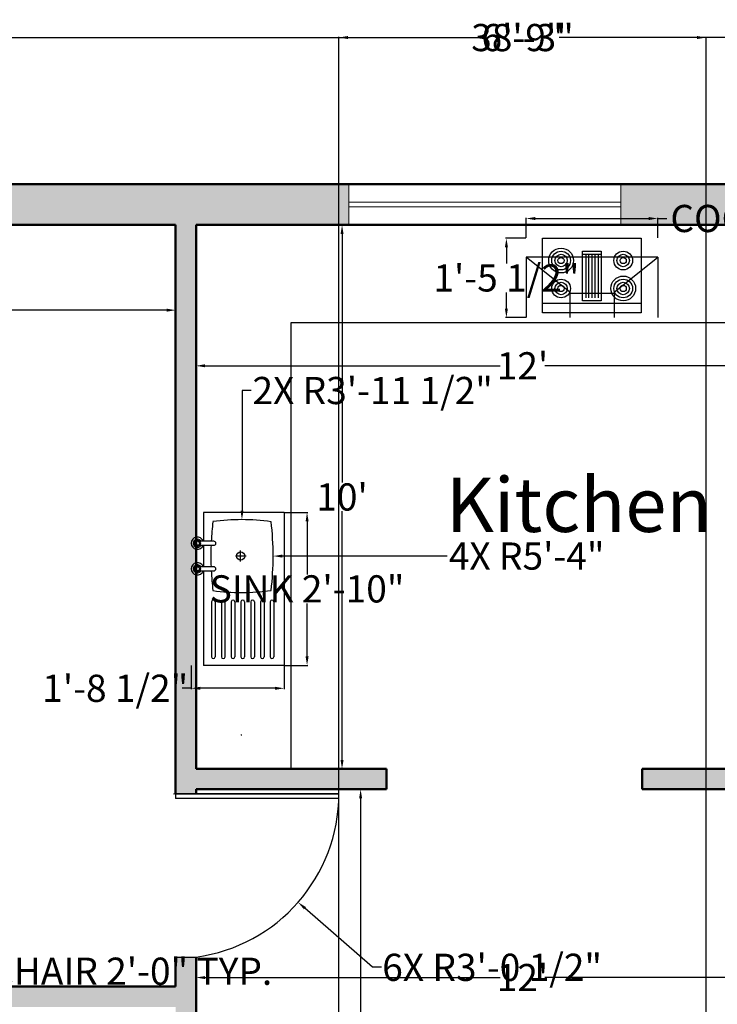
# Model space of a CAD drawing. Units: inches. Extents: x 2436 to 2989, y 5527 to 6207.
# Tile 4 of 5: x 2605 to 2759, y 5989 to 6207. Entities that reach past the tile are written whole.
import ezdxf

# ---------------------------------------------------------------- set-up
doc = ezdxf.new("R2010")
doc.units = ezdxf.units.IN
doc.header["$MEASUREMENT"] = 0
for name, color, linetype, lineweight in [('A-ANNO-DIMS', 2, 'Continuous', 18), ('A-AREA-IDEN', 7, 'Continuous', 25), ('A-DOOR', 3, 'Continuous', 25), ('A-EQPM', 8, 'Continuous', 25), ('A-FLOR-CASE', 9, 'Continuous', 25), ('A-FLOR-FIXT', 8, 'Continuous', 25), ('A-GLAZ', 4, 'Continuous', 18), ('A-WALL', 7, 'Continuous', 50), ('A-WALL-PATT', 252, 'Continuous', 13)]:
    doc.layers.add(name, color=color, linetype=linetype, lineweight=lineweight)
doc.styles.get("Standard").update_dxf_attribs({"font": 'arial.ttf'})
doc.dimstyles.get("Standard").update_dxf_attribs({"dimtxt": 6, "dimasz": 2, "dimexe": 0.18, "dimexo": 0.0625, "dimgap": 0.09, "dimtad": 0, "dimtih": 1, "dimtoh": 1, "dimdec": 0, "dimzin": 0, "dimdsep": 46, "dimlunit": 3, "dimtxsty": 'Standard', "dimcen": 0.09, "dimadec": 0, "dimazin": 0, "dimtfac": 1, "dimtdec": 0, "dimtofl": 0, "dimtmove": 0, "dimatfit": 3, "dimfxl": 1, "dimtolj": 1, "dimtzin": 0, "dimarcsym": 0})

# ---------------------------------------------------------------- blocks, each defined once
blk = doc.blocks.new('*D4')
at = {"layer": 'A-ANNO-DIMS', "color": 0, "lineweight": -2, "transparency": 16777216}
for p, q in [((2495.39, 6161.17), (2495.39, 6142.26)), ((2639.39, 6161.17), (2639.39, 6142.26)), ((2497.39, 6142.44), (2562.49, 6142.44)), ((2637.39, 6142.44), (2572.29, 6142.44))]:
    blk.add_line(p, q, dxfattribs=at)
at = {"layer": 'A-ANNO-DIMS', "color": 0, "transparency": 16777216}
for points in [[(2497.39, 6142.77), (2497.39, 6142.1), (2495.39, 6142.44)], [(2637.39, 6142.77), (2637.39, 6142.1), (2639.39, 6142.44)]]:
    blk.add_solid(points, dxfattribs=at)
at = {"layer": 'Defpoints', "color": 0, "transparency": 16777216}
for p in [(2495.39, 6161.23), (2639.39, 6161.23), (2639.39, 6142.44)]:
    blk.add_point(p, dxfattribs=at)
at = {"layer": 'A-ANNO-DIMS', "color": 0, "transparency": 16777216, "insert": (2567.39, 6142.44), "char_height": 6, "attachment_point": 5}
blk.add_mtext("\\A1;12'", dxfattribs=at)
blk = doc.blocks.new('*D5')
at = {"layer": 'A-ANNO-DIMS', "color": 0, "lineweight": -2, "transparency": 16777216}
for p, q in [((2643.89, 6161.17), (2643.89, 6129.98)), ((2787.89, 6161.17), (2787.89, 6129.98)), ((2645.89, 6130.16), (2710.99, 6130.16)), ((2785.89, 6130.16), (2720.79, 6130.16))]:
    blk.add_line(p, q, dxfattribs=at)
at = {"layer": 'A-ANNO-DIMS', "color": 0, "transparency": 16777216}
for points in [[(2645.89, 6130.5), (2645.89, 6129.83), (2643.89, 6130.16)], [(2785.89, 6130.5), (2785.89, 6129.83), (2787.89, 6130.16)]]:
    blk.add_solid(points, dxfattribs=at)
at = {"layer": 'Defpoints', "color": 0, "transparency": 16777216}
for p in [(2643.89, 6161.23), (2787.89, 6161.23), (2787.89, 6130.16)]:
    blk.add_point(p, dxfattribs=at)
at = {"layer": 'A-ANNO-DIMS', "color": 0, "transparency": 16777216, "insert": (2715.89, 6130.16), "char_height": 6, "attachment_point": 5}
blk.add_mtext("\\A1;12'", dxfattribs=at)
blk = doc.blocks.new('*D6')
at = {"layer": 'A-ANNO-DIMS', "color": 0, "lineweight": -2, "transparency": 16777216}
for p, q in [((2643.95, 6161.23), (2676.27, 6161.23)), ((2676.09, 6159.23), (2676.09, 6104.39)), ((2676.09, 6043.23), (2676.09, 6098.08)), ((2643.95, 6041.23), (2676.27, 6041.23))]:
    blk.add_line(p, q, dxfattribs=at)
at = {"layer": 'A-ANNO-DIMS', "color": 0, "transparency": 16777216}
for points in [[(2675.76, 6159.23), (2676.43, 6159.23), (2676.09, 6161.23)], [(2675.76, 6043.23), (2676.43, 6043.23), (2676.09, 6041.23)]]:
    blk.add_solid(points, dxfattribs=at)
at = {"layer": 'Defpoints', "color": 0, "transparency": 16777216}
for p in [(2643.89, 6161.23), (2643.89, 6041.23), (2676.09, 6041.23)]:
    blk.add_point(p, dxfattribs=at)
at = {"layer": 'A-ANNO-DIMS', "color": 0, "transparency": 16777216, "insert": (2676.09, 6101.23), "char_height": 6, "attachment_point": 5}
blk.add_mtext("\\A1;10'", dxfattribs=at)
blk = doc.blocks.new('*D19')
at = {"layer": 'A-ANNO-DIMS', "color": 0, "lineweight": -2, "transparency": 16777216}
for p, q in [((2667.17, 6036.73), (2680.37, 6036.73)), ((2680.19, 6034.73), (2680.19, 5949.89)), ((2680.19, 5858.73), (2680.19, 5943.58)), ((2667.17, 5856.73), (2680.37, 5856.73))]:
    blk.add_line(p, q, dxfattribs=at)
at = {"layer": 'A-ANNO-DIMS', "color": 0, "transparency": 16777216}
for points in [[(2679.86, 6034.73), (2680.52, 6034.73), (2680.19, 6036.73)], [(2679.86, 5858.73), (2680.52, 5858.73), (2680.19, 5856.73)]]:
    blk.add_solid(points, dxfattribs=at)
at = {"layer": 'Defpoints', "color": 0, "transparency": 16777216}
for p in [(2667.11, 6036.73), (2667.11, 5856.73), (2680.19, 5856.73)]:
    blk.add_point(p, dxfattribs=at)
at = {"layer": 'A-ANNO-DIMS', "color": 0, "transparency": 16777216, "insert": (2680.19, 5946.73), "char_height": 6, "attachment_point": 5}
blk.add_mtext("\\A1;15'", dxfattribs=at)
blk = doc.blocks.new('*D20')
at = {"layer": 'A-ANNO-DIMS', "color": 0, "lineweight": -2, "transparency": 16777216}
for p, q in [((2643.89, 5989.83), (2643.89, 5995.38)), ((2787.89, 5989.83), (2787.89, 5995.38)), ((2645.89, 5995.2), (2710.99, 5995.2)), ((2785.89, 5995.2), (2720.79, 5995.2))]:
    blk.add_line(p, q, dxfattribs=at)
at = {"layer": 'A-ANNO-DIMS', "color": 0, "transparency": 16777216}
for points in [[(2645.89, 5995.53), (2645.89, 5994.87), (2643.89, 5995.2)], [(2785.89, 5995.53), (2785.89, 5994.87), (2787.89, 5995.2)]]:
    blk.add_solid(points, dxfattribs=at)
at = {"layer": 'Defpoints', "color": 0, "transparency": 16777216}
for p in [(2787.89, 5995.2), (2643.89, 5989.77), (2787.89, 5989.77)]:
    blk.add_point(p, dxfattribs=at)
at = {"layer": 'A-ANNO-DIMS', "color": 0, "transparency": 16777216, "insert": (2715.89, 5995.2), "char_height": 6, "attachment_point": 5}
blk.add_mtext("\\A1;12'", dxfattribs=at)
blk = doc.blocks.new('chimmne')
for p, q in [((17.89, 6.07), (-18.11, 6.07)), ((-18.11, 6.07), (-18.11, -10.43)), ((-6.16, -3.43), (-18.11, 6.07)), ((5.94, -3.43), (17.89, 6.07)), ((17.89, 6.07), (17.89, -10.43)), ((-6.16, -3.43), (-6.16, -10.43)), ((5.94, -3.82), (-6.16, -3.82)), ((5.94, -3.43), (5.94, -10.43))]:
    blk.add_line(p, q)
for points in [[(-13.61, -9.12), (-13.61, 11.28), (13.39, 11.28), (13.39, -9.12)], [(-2.66, -5.87), (-2.66, 7.73), (2.44, 7.73), (2.44, -5.87)]]:
    blk.add_lwpolyline(points, close=True)
for points in [[(-2.66, 6.88), (2.44, 6.88)], [(-1.81, 6.88), (-1.81, -5.02)], [(-0.96, -5.02), (-0.96, 6.88)], [(-0.11, 6.88), (-0.11, -5.02)], [(0.74, -5.02), (0.74, 6.88)], [(1.59, 6.88), (1.59, -5.02)], [(13.39, -6.57), (-13.61, -6.57)]]:
    blk.add_lwpolyline(points)
for centre, radius in [((-8.55, 5.18), 3.4), ((-8.55, 5.18), 2.55), ((-8.55, 5.18), 1.7), ((-8.55, 5.18), 0.85), ((8.44, 5.18), 2.55), ((8.44, 5.18), 1.7), ((8.44, 5.18), 0.85), ((-8.55, -2.47), 2.55), ((8.44, -2.47), 3.4), ((8.44, -2.47), 2.55), ((-8.55, -2.47), 1.7), ((-8.55, -2.47), 0.85), ((8.44, -2.47), 1.7), ((8.44, -2.47), 0.85)]:
    blk.add_circle(centre, radius)
blk = doc.blocks.new('A$C799204C7')
for p, q in [((0, 34.2), (17.99, 34.2)), ((0, 0), (0, 34.2)), ((17.99, 13.08), (17.99, 34.2)), ((2.32, 20.01), (2.32, 32.27)), ((3.13, 20.01), (3.13, 32.27)), ((4.48, 20.01), (4.48, 32.27)), ((5.29, 20.01), (5.29, 32.27)), ((6.64, 20.01), (6.64, 32.27)), ((7.45, 20.01), (7.45, 32.27)), ((8.85, 20.01), (8.85, 32.27)), ((9.66, 20.01), (9.66, 32.27)), ((11.01, 20.01), (11.01, 32.27)), ((11.82, 20.01), (11.82, 32.27)), ((13.22, 20.01), (13.22, 32.27)), ((14.03, 20.01), (14.03, 32.27)), ((15.42, 20.01), (15.42, 32.27)), ((16.24, 20.01), (16.24, 32.27)), ((18.59, 13.08), (15.71, 13.08)), ((15.71, 12.17), (18.59, 12.17)), ((17.99, 7.36), (17.99, 12.17)), ((8.52, 9.77), (10.9, 9.77)), ((9.73, 11), (9.73, 8.54)), ((18.59, 7.36), (15.71, 7.36)), ((15.71, 6.45), (18.59, 6.45)), ((17.99, 0), (17.99, 6.45)), ((0, 0), (17.99, 0))]:
    blk.add_line(p, q)
for centre, radius in [((19.38, 12.62), 0.684), ((19.38, 12.62), 0.456), ((9.7, 9.77), 0.916), ((19.38, 6.91), 0.684), ((19.38, 6.91), 0.456)]:
    blk.add_circle(centre, radius)
for centre, radius, start, end in [((2.72, 32.27), 0.407, 0, 180), ((4.88, 32.27), 0.407, 0, 180), ((7.05, 32.27), 0.407, 0, 180), ((9.25, 32.27), 0.407, 0, 180), ((11.42, 32.27), 0.407, 0, 180), ((13.62, 32.27), 0.407, 0, 180), ((15.83, 32.27), 0.407, 0, 180), ((2.72, 20.01), 0.407, 180, 0), ((4.88, 20.01), 0.407, 180, 0), ((7.05, 20.01), 0.407, 180, 0), ((9.25, 20.01), 0.407, 180, 0), ((11.42, 20.01), 0.407, 180, 0), ((13.62, 20.01), 0.407, 180, 0), ((15.83, 20.01), 0.407, 180, 0), ((9.53, -30.19), 48.1, 82.3437, 97.8966), ((67.33, 9.77), 64.88, 173.1952, 186.8048), ((-48.51, 9.77), 64.88, 2.9208, 6.8048), ((19.38, 12.62), 1.37, 199.6514, 160.3603), ((19.38, 12.62), 0.911, 210.3431, 149.7554), ((15.71, 12.62), 0.456, 90, 270), ((-48.51, 9.77), 64.88, 357.8723, 2.115), ((15.71, 6.91), 0.456, 90, 270), ((19.38, 6.91), 1.37, 199.6514, 160.3603), ((19.38, 6.91), 0.911, 210.3431, 149.7554), ((-48.51, 9.77), 64.88, 353.1952, 357.0665), ((9.53, 49.73), 48.1, 262.1034, 277.6563)]:
    blk.add_arc(centre, radius, start, end)
blk = doc.blocks.new('WINDOW-60IN')
for p, q in [((0, 9), (0, 0)), ((60, 9), (0, 9)), ((60, 0), (60, 9)), ((60, 5), (0, 5)), ((0, 4), (60, 4)), ((0, 0), (60, 0))]:
    blk.add_line(p, q)
blk = doc.blocks.new('*D34')
at = {"layer": 'A-ANNO-DIMS', "color": 0, "lineweight": -2, "transparency": 16777216}
for p, q in [((2553.14, 6000.14), (2553.14, 5996.42)), ((2577.11, 6000.14), (2577.11, 5996.42)), ((2555.14, 5996.6), (2575.11, 5996.6)), ((2577.11, 5996.6), (2579.11, 5996.6))]:
    blk.add_line(p, q, dxfattribs=at)
at = {"layer": 'A-ANNO-DIMS', "color": 0, "transparency": 16777216}
for points in [[(2555.14, 5996.94), (2555.14, 5996.27), (2553.14, 5996.6)], [(2575.11, 5996.94), (2575.11, 5996.27), (2577.11, 5996.6)]]:
    blk.add_solid(points, dxfattribs=at)
at = {"layer": 'Defpoints', "color": 0, "transparency": 16777216}
for p in [(2553.14, 6000.2), (2577.11, 6000.2), (2577.11, 5996.6)]:
    blk.add_point(p, dxfattribs=at)
at = {"layer": 'A-ANNO-DIMS', "color": 0, "transparency": 16777216, "insert": (2621.18, 5996.6), "char_height": 6, "attachment_point": 5}
blk.add_mtext('\\A1;ARMCHAIR 2\'-0" TYP.', dxfattribs=at)
blk = doc.blocks.new('*D44')
at = {"layer": 'A-ANNO-DIMS', "color": 0, "lineweight": -2, "transparency": 16777216}
for p, q in [((2716.7, 6158.37), (2716.7, 6162.84)), ((2718.7, 6162.66), (2743.72, 6162.66)), ((2745.72, 6158.37), (2745.72, 6162.84)), ((2745.72, 6162.66), (2747.72, 6162.66))]:
    blk.add_line(p, q, dxfattribs=at)
at = {"layer": 'A-ANNO-DIMS', "color": 0, "transparency": 16777216}
for points in [[(2718.7, 6162.99), (2718.7, 6162.32), (2716.7, 6162.66)], [(2743.72, 6162.99), (2743.72, 6162.32), (2745.72, 6162.66)]]:
    blk.add_solid(points, dxfattribs=at)
at = {"layer": 'Defpoints', "color": 0, "transparency": 16777216}
for p in [(2745.72, 6162.66), (2716.7, 6158.3), (2745.72, 6158.3)]:
    blk.add_point(p, dxfattribs=at)
at = {"layer": 'A-ANNO-DIMS', "color": 0, "transparency": 16777216, "insert": (2777.87, 6162.66), "char_height": 6, "attachment_point": 5}
blk.add_mtext('\\A1;COOKTOP 2\'-5"', dxfattribs=at)
blk = doc.blocks.new('*D45')
at = {"layer": 'A-ANNO-DIMS', "color": 0, "lineweight": -2, "transparency": 16777216}
for p, q in [((2716.63, 6158.3), (2712.16, 6158.3)), ((2712.34, 6156.3), (2712.34, 6152.75)), ((2712.34, 6142.8), (2712.34, 6146.36)), ((2716.63, 6140.8), (2712.16, 6140.8))]:
    blk.add_line(p, q, dxfattribs=at)
at = {"layer": 'A-ANNO-DIMS', "color": 0, "transparency": 16777216}
for points in [[(2712.01, 6156.3), (2712.68, 6156.3), (2712.34, 6158.3)], [(2712.01, 6142.8), (2712.68, 6142.8), (2712.34, 6140.8)]]:
    blk.add_solid(points, dxfattribs=at)
at = {"layer": 'Defpoints', "color": 0, "transparency": 16777216}
for p in [(2712.34, 6158.3), (2716.7, 6158.3), (2716.7, 6140.8)]:
    blk.add_point(p, dxfattribs=at)
at = {"layer": 'A-ANNO-DIMS', "color": 0, "transparency": 16777216, "insert": (2712.34, 6149.55), "char_height": 6, "attachment_point": 5}
blk.add_mtext('\\A1;1\'-5 1/2"', dxfattribs=at)
blk = doc.blocks.new('*D46')
at = {"layer": 'A-ANNO-DIMS', "color": 0, "lineweight": -2, "transparency": 16777216}
for p, q in [((2663.38, 6097.83), (2668.56, 6097.83)), ((2668.38, 6095.83), (2668.38, 6084.15)), ((2668.38, 6066.08), (2668.38, 6077.76)), ((2663.38, 6064.08), (2668.56, 6064.08))]:
    blk.add_line(p, q, dxfattribs=at)
at = {"layer": 'A-ANNO-DIMS', "color": 0, "transparency": 16777216}
for points in [[(2668.05, 6095.83), (2668.72, 6095.83), (2668.38, 6097.83)], [(2668.05, 6066.08), (2668.72, 6066.08), (2668.38, 6064.08)]]:
    blk.add_solid(points, dxfattribs=at)
at = {"layer": 'Defpoints', "color": 0, "transparency": 16777216}
for p in [(2663.32, 6097.83), (2663.32, 6064.08), (2668.38, 6064.08)]:
    blk.add_point(p, dxfattribs=at)
at = {"layer": 'A-ANNO-DIMS', "color": 0, "transparency": 16777216, "insert": (2668.38, 6080.95), "char_height": 6, "attachment_point": 5}
blk.add_mtext('\\A1;SINK 2\'-10"', dxfattribs=at)
blk = doc.blocks.new('*D47')
at = {"layer": 'A-ANNO-DIMS', "color": 0, "lineweight": -2, "transparency": 16777216}
for p, q in [((2642.85, 6064.02), (2642.85, 6058.84)), ((2663.32, 6064.02), (2663.32, 6058.84)), ((2642.85, 6059.02), (2640.85, 6059.02)), ((2661.32, 6059.02), (2644.85, 6059.02))]:
    blk.add_line(p, q, dxfattribs=at)
at = {"layer": 'A-ANNO-DIMS', "color": 0, "transparency": 16777216}
for points in [[(2644.85, 6059.35), (2644.85, 6058.68), (2642.85, 6059.02)], [(2661.32, 6059.35), (2661.32, 6058.68), (2663.32, 6059.02)]]:
    blk.add_solid(points, dxfattribs=at)
at = {"layer": 'Defpoints', "color": 0, "transparency": 16777216}
for p in [(2642.85, 6064.08), (2663.32, 6064.08), (2642.85, 6059.02)]:
    blk.add_point(p, dxfattribs=at)
at = {"layer": 'A-ANNO-DIMS', "color": 0, "transparency": 16777216, "insert": (2626.07, 6059.02), "char_height": 6, "attachment_point": 5}
blk.add_mtext('\\A1;1\'-8 1/2"', dxfattribs=at)
blk = doc.blocks.new('*D48')
at = {"layer": 'A-ANNO-DIMS', "color": 0, "lineweight": -2, "transparency": 16777216}
for p, q in [((2486.39, 6170.29), (2486.39, 6202.76)), ((2488.39, 6202.58), (2705.49, 6202.58)), ((2943.39, 6202.58), (2726.28, 6202.58)), ((2945.39, 6080.73), (2945.39, 6202.76))]:
    blk.add_line(p, q, dxfattribs=at)
at = {"layer": 'A-ANNO-DIMS', "color": 0, "transparency": 16777216}
for points in [[(2488.39, 6202.92), (2488.39, 6202.25), (2486.39, 6202.58)], [(2943.39, 6202.92), (2943.39, 6202.25), (2945.39, 6202.58)]]:
    blk.add_solid(points, dxfattribs=at)
at = {"layer": 'Defpoints', "color": 0, "transparency": 16777216}
for p in [(2945.39, 6202.58), (2486.39, 6170.23), (2945.39, 6080.66)]:
    blk.add_point(p, dxfattribs=at)
at = {"layer": 'A-ANNO-DIMS', "color": 0, "transparency": 16777216, "insert": (2715.89, 6202.58), "char_height": 6, "attachment_point": 5}
blk.add_mtext('\\A1;38\'-3"', dxfattribs=at)
blk = doc.blocks.new('*D49')
at = {"layer": 'A-ANNO-DIMS', "color": 0, "lineweight": -2, "transparency": 16777216}
for p, q in [((2486.33, 6170.23), (2453.86, 6170.23)), ((2454.04, 6168.23), (2454.04, 5851.68)), ((2454.04, 5528.73), (2454.04, 5845.29)), ((2675.33, 5526.73), (2453.86, 5526.73))]:
    blk.add_line(p, q, dxfattribs=at)
at = {"layer": 'A-ANNO-DIMS', "color": 0, "transparency": 16777216}
for points in [[(2453.7, 6168.23), (2454.37, 6168.23), (2454.04, 6170.23)], [(2453.7, 5528.73), (2454.37, 5528.73), (2454.04, 5526.73)]]:
    blk.add_solid(points, dxfattribs=at)
at = {"layer": 'Defpoints', "color": 0, "transparency": 16777216}
for p in [(2486.39, 6170.23), (2454.04, 5526.73), (2675.39, 5526.73)]:
    blk.add_point(p, dxfattribs=at)
at = {"layer": 'A-ANNO-DIMS', "color": 0, "transparency": 16777216, "insert": (2454.04, 5848.48), "char_height": 6, "attachment_point": 5}
blk.add_mtext('\\A1;53\'-7 1/2"', dxfattribs=at)
blk = doc.blocks.new('*D51')
at = {"layer": 'A-ANNO-DIMS', "color": 0, "lineweight": -2, "transparency": 16777216}
for p, q in [((2675.39, 5526.79), (2675.39, 6202.76)), ((2677.39, 6202.58), (2707.81, 6202.58)), ((2754.39, 6202.58), (2723.97, 6202.58)), ((2756.39, 5526.79), (2756.39, 6202.76))]:
    blk.add_line(p, q, dxfattribs=at)
at = {"layer": 'A-ANNO-DIMS', "color": 0, "transparency": 16777216}
for points in [[(2677.39, 6202.92), (2677.39, 6202.25), (2675.39, 6202.58)], [(2754.39, 6202.92), (2754.39, 6202.25), (2756.39, 6202.58)]]:
    blk.add_solid(points, dxfattribs=at)
at = {"layer": 'Defpoints', "color": 0, "transparency": 16777216}
for p in [(2756.39, 6202.58), (2675.39, 5526.73), (2756.39, 5526.73)]:
    blk.add_point(p, dxfattribs=at)
at = {"layer": 'A-ANNO-DIMS', "color": 0, "transparency": 16777216, "insert": (2715.89, 6202.58), "char_height": 6, "attachment_point": 5}
blk.add_mtext('\\A1;6\'-9"', dxfattribs=at)
blk = doc.blocks.new('*D54')
at = {"layer": 'A-ANNO-DIMS', "color": 0, "lineweight": -2, "transparency": 16777216}
for p, q in [((2638.98, 6035.73), (2639.16, 6035.73)), ((2639.07, 6035.64), (2639.07, 6035.82)), ((2682.8, 5997.46), (2667.91, 6010.5)), ((2684.8, 5997.46), (2682.8, 5997.46))]:
    blk.add_line(p, q, dxfattribs=at)
at = {"layer": 'A-ANNO-DIMS', "color": 0, "transparency": 16777216}
blk.add_solid([(2668.13, 6010.75), (2667.69, 6010.25), (2666.4, 6011.81)], dxfattribs=at)
at = {"layer": 'Defpoints', "color": 0, "transparency": 16777216}
for p in [(2639.07, 6035.73), (2666.4, 6011.81)]:
    blk.add_point(p, dxfattribs=at)
at = {"layer": 'A-ANNO-DIMS', "color": 0, "transparency": 16777216, "insert": (2709.19, 5997.46), "char_height": 6, "attachment_point": 5}
blk.add_mtext('\\A1;6X R3\'-0 1/2"', dxfattribs=at)
blk = doc.blocks.new('*D56')
at = {"layer": 'A-ANNO-DIMS', "color": 0, "lineweight": -2, "transparency": 16777216}
for p, q in [((2596.78, 6088.19), (2596.96, 6088.19)), ((2596.87, 6088.1), (2596.87, 6088.28)), ((2699.31, 6088.19), (2662.89, 6088.19))]:
    blk.add_line(p, q, dxfattribs=at)
at = {"layer": 'A-ANNO-DIMS', "color": 0, "transparency": 16777216}
blk.add_solid([(2662.89, 6088.52), (2662.89, 6087.85), (2660.89, 6088.19)], dxfattribs=at)
at = {"layer": 'Defpoints', "color": 0, "transparency": 16777216}
for p in [(2596.87, 6088.19), (2660.89, 6088.19)]:
    blk.add_point(p, dxfattribs=at)
at = {"layer": 'A-ANNO-DIMS', "color": 0, "transparency": 16777216, "insert": (2716.81, 6088.19), "char_height": 6, "attachment_point": 5}
blk.add_mtext('\\A1;4X R5\'-4"', dxfattribs=at)
blk = doc.blocks.new('*D57')
at = {"layer": 'A-ANNO-DIMS', "color": 0, "lineweight": -2, "transparency": 16777216}
for p, q in [((2654.08, 6124.71), (2654.03, 6098.22)), ((2656.08, 6124.71), (2654.08, 6124.71)), ((2653.83, 6048.75), (2654.01, 6048.75)), ((2653.92, 6048.66), (2653.92, 6048.84))]:
    blk.add_line(p, q, dxfattribs=at)
at = {"layer": 'A-ANNO-DIMS', "color": 0, "transparency": 16777216}
blk.add_solid([(2653.69, 6098.22), (2654.36, 6098.22), (2654.02, 6096.22)], dxfattribs=at)
at = {"layer": 'Defpoints', "color": 0, "transparency": 16777216}
for p in [(2654.02, 6096.22), (2653.92, 6048.75)]:
    blk.add_point(p, dxfattribs=at)
at = {"layer": 'A-ANNO-DIMS', "color": 0, "transparency": 16777216, "insert": (2682.84, 6124.71), "char_height": 6, "attachment_point": 5}
blk.add_mtext('\\A1;2X R3\'-11 1/2"', dxfattribs=at)

msp = doc.modelspace()

# ---------------------------------------------------------------- hatches: boundary and pattern name
at = {"layer": 'A-WALL-PATT'}
h = msp.add_hatch(color=256, dxfattribs=at)
h.dxf.hatch_style = 1
h.paths.add_polyline_path([(2533.49, 6170.23), (2486.39, 6170.23), (2486.39, 6124.33), (2495.39, 6124.33), (2495.39, 6161.23), (2533.49, 6161.23)])
h.paths.add_polyline_path([(2677.58, 6170.23), (2593.49, 6170.23), (2593.49, 6161.23), (2639.39, 6161.23), (2639.39, 6035.73), (2639.39, 6035.73), (2643.89, 6035.73), (2643.89, 6036.73), (2685.89, 6036.73), (2685.89, 6041.23), (2643.89, 6041.23), (2643.89, 6161.23), (2677.58, 6161.23)])
h.paths.add_polyline_path([(2792.39, 6170.23), (2737.58, 6170.23), (2737.58, 6161.23), (2787.89, 6161.23), (2787.89, 6084.23), (2792.39, 6084.23), (2792.39, 6161.23), (2936.39, 6161.23), (2936.39, 6071.23), (2840.39, 6071.23), (2840.39, 6047.23), (2792.39, 6047.23), (2792.39, 6048.23), (2787.89, 6048.23), (2787.89, 6047.23), (2787.89, 6041.23), (2742.3, 6041.23), (2742.3, 6036.73), (2787.89, 6036.73), (2787.89, 6035.73), (2792.39, 6035.73), (2792.39, 6042.73), (2840.39, 6042.73), (2840.39, 5945.23), (2792.39, 5945.23), (2792.39, 6003.73), (2787.89, 6003.73), (2787.89, 5893.73), (2792.39, 5893.73), (2792.39, 5940.73), (2845.89, 5940.73), (2845.89, 5945.23), (2844.89, 5945.23), (2844.89, 6047.23), (2844.89, 6066.73), (2936.39, 6066.73), (2936.39, 6024.33), (2945.39, 6024.33), (2945.39, 6080.66), (2940.89, 6080.66), (2940.89, 6165.73), (2792.39, 6165.73)])
h.paths.add_polyline_path([(2945.39, 6000.33), (2936.39, 6000.33), (2936.39, 5945.23), (2881.89, 5945.23), (2881.89, 5940.73), (2936.39, 5940.73), (2936.39, 5901.74), (2945.39, 5901.74)], flags=17)
h.paths.add_polyline_path([(2945.39, 5841.74), (2936.39, 5841.74), (2936.39, 5796.73), (2792.39, 5796.73), (2792.39, 5857.73), (2787.89, 5857.73), (2787.89, 5856.73), (2786.89, 5856.73), (2786.89, 5852.23), (2787.89, 5852.23), (2787.89, 5792.23), (2892.89, 5792.23), (2892.89, 5760.78), (2901.89, 5760.78), (2901.89, 5792.23), (2945.39, 5792.23)])
h.paths.add_polyline_path([(2495.39, 5880.74), (2486.39, 5880.74), (2486.39, 5787.73), (2525.39, 5787.73), (2525.39, 5761.57), (2534.39, 5761.57), (2534.39, 5792.23), (2639.39, 5792.23), (2639.39, 5733.23), (2643.89, 5733.23), (2643.89, 5852.23), (2750.89, 5852.23), (2750.89, 5856.73), (2643.89, 5856.73), (2643.89, 5857.73), (2639.39, 5857.73), (2639.39, 5796.73), (2495.39, 5796.73)])
h.paths.add_polyline_path([(2495.39, 6064.33), (2486.39, 6064.33), (2486.39, 5940.74), (2495.39, 5940.74), (2495.39, 5988.73), (2639.39, 5988.73), (2639.39, 5893.73), (2643.89, 5893.73), (2643.89, 5999.73), (2639.39, 5999.73), (2639.39, 5993.23), (2495.39, 5993.23)])
h.paths.add_polyline_path([(2682.14, 5696.23), (2643.89, 5696.23), (2643.89, 5697.23), (2639.39, 5697.23), (2639.39, 5696.23), (2558.39, 5696.23), (2534.39, 5696.23), (2534.39, 5737.57), (2525.39, 5737.57), (2525.39, 5687.23), (2534.39, 5687.23), (2558.39, 5687.23), (2643.89, 5687.23), (2682.14, 5687.23)])
h.paths.add_polyline_path([(2901.89, 5736.78), (2892.89, 5736.78), (2892.89, 5696.23), (2868.89, 5696.23), (2751.89, 5696.23), (2751.89, 5687.23), (2787.89, 5687.23), (2787.89, 5567.23), (2792.39, 5567.23), (2792.39, 5687.23), (2868.89, 5687.23), (2892.89, 5687.23), (2901.89, 5687.23)])
h.paths.add_polyline_path([(2643.89, 5687.23), (2639.39, 5687.23), (2639.39, 5567.23), (2643.89, 5567.23)])
h.paths.add_polyline_path([(2787.89, 5567.23), (2643.89, 5567.23), (2643.89, 5562.73), (2787.89, 5562.73)])
h.paths.add_polyline_path([(2643.89, 5567.23), (2639.39, 5567.23), (2639.39, 5562.73), (2643.89, 5562.73)])
h.paths.add_polyline_path([(2792.39, 5567.23), (2787.89, 5567.23), (2787.89, 5562.73), (2792.39, 5562.73)])

# ---------------------------------------------------------------- linework, layer by layer
at = {"layer": 'A-DOOR'}
for p, q in [((2639.39, 6036.73), (2639.39, 6035.73)), ((2639.39, 6035.73), (2675.39, 6035.73)), ((2675.39, 6035.73), (2639.39, 6035.73)), ((2639.39, 6035.73), (2639.39, 6034.73)), ((2675.39, 6034.73), (2639.39, 6034.73)), ((2639.39, 5999.73), (2643.89, 5999.73))]:
    msp.add_line(p, q, dxfattribs=at)
msp.add_arc((2639.07, 6035.73), 36.32, 277.6281, 360, dxfattribs=at)
at = {"layer": 'A-FLOR-CASE'}
for p, q in [((2664.89, 6041.23), (2664.89, 6139.73)), ((2664.89, 6139.73), (2787.89, 6139.73))]:
    msp.add_line(p, q, dxfattribs=at)
at = {"layer": 'A-WALL'}
for p, q in [((2486.39, 6170.23), (2792.39, 6170.23)), ((2495.39, 6161.23), (2639.39, 6161.23)), ((2639.39, 6161.23), (2639.39, 6035.73)), ((2643.89, 6161.23), (2643.89, 6041.23)), ((2643.89, 6161.23), (2787.89, 6161.23)), ((2643.89, 6041.23), (2685.89, 6041.23)), ((2643.89, 6041.23), (2685.89, 6041.23)), ((2685.89, 6041.23), (2685.89, 6036.73)), ((2742.3, 6036.73), (2742.3, 6041.23)), ((2742.3, 6041.23), (2787.89, 6041.23)), ((2643.89, 6036.73), (2685.89, 6036.73)), ((2643.89, 6036.73), (2643.89, 6035.73)), ((2742.3, 6036.73), (2787.89, 6036.73)), ((2639.39, 5993.23), (2639.39, 5999.73)), ((2643.89, 5999.73), (2643.89, 5893.73)), ((2495.39, 5993.23), (2639.39, 5993.23))]:
    msp.add_line(p, q, dxfattribs=at)

# ---------------------------------------------------------------- block references
at = {"layer": 'A-EQPM', "xscale": 0.8061586867187187, "yscale": 0.8061586867187187, "zscale": 0.8061586867187187}
msp.add_blockref('chimmne', (2731.3, 6149.21), dxfattribs=at)
at = {"layer": 'A-FLOR-FIXT', "xscale": 0.9869076798868125, "yscale": 0.9869076798868125, "zscale": 0.9869076798868125, "rotation": 180}
msp.add_blockref('A$C799204C7', (2663.32, 6097.83), dxfattribs=at)
at = {"layer": 'A-GLAZ'}
msp.add_blockref('WINDOW-60IN', (2677.58, 6161.23), dxfattribs=at)

# ---------------------------------------------------------------- texts
at = {"layer": 'A-AREA-IDEN', "insert": (2699.02, 6105.51), "char_height": 12, "attachment_point": 1}
msp.add_mtext_dynamic_manual_height_columns('Kitchen', width=75.4838, gutter_width=1, heights=[0], dxfattribs=at)

# ---------------------------------------------------------------- dimensions: what is measured, and where the dimension line sits
at = {"layer": 'A-ANNO-DIMS'}
for base, p1, p2, override, picture, middle in [((2945.39, 6202.58), (2486.39, 6170.23), (2945.39, 6080.66), {"dimdec": 1, "dimlfac": 1, "dimrnd": 0, "dimzin": 1, "dimdsep": 46, "dimlunit": 4, "dimfrac": 2}, '*D48', (2715.89, 6202.58)), ((2756.39, 6202.58), (2675.39, 5526.73), (2756.39, 5526.73), {"dimdec": 1, "dimlfac": 1, "dimrnd": 0, "dimzin": 1, "dimdsep": 46, "dimlunit": 4, "dimfrac": 2}, '*D51', (2715.89, 6202.58)), ((2639.39, 6142.44), (2495.39, 6161.23), (2639.39, 6161.23), {"dimclrd": 0, "dimclre": 0, "dimclrt": 0}, '*D4', (2567.39, 6142.44)), ((2787.89, 6130.16), (2643.89, 6161.23), (2787.89, 6161.23), {"dimclrd": 0, "dimclre": 0, "dimclrt": 0}, '*D5', (2715.89, 6130.16)), ((2787.89, 5995.2), (2643.89, 5989.77), (2787.89, 5989.77), {"dimclrd": 0, "dimclre": 0, "dimclrt": 0}, '*D20', (2715.89, 5995.2))]:
    dim = msp.add_linear_dim(base=base, p1=p1, p2=p2, dimstyle='Standard', override=override, dxfattribs=at)
    dim.commit()
    dim.dimension.update_dxf_attribs({"geometry": picture, "text_midpoint": middle})
for base, p1, p2, text, picture, middle in [((2745.72, 6162.66), (2716.7, 6158.3), (2745.72, 6158.3), 'COOKTOP <>', '*D44', (2777.87, 6162.66)), ((2577.11, 5996.6), (2553.14, 6000.2), (2577.11, 6000.2), 'ARMCHAIR <> TYP.', '*D34', (2621.18, 5996.6))]:
    dim = msp.add_linear_dim(base=base, p1=p1, p2=p2, text=text, dimstyle='Standard', override={"dimdec": 1, "dimlfac": 1, "dimrnd": 0, "dimzin": 1, "dimdsep": 46, "dimlunit": 4, "dimfrac": 2}, dxfattribs=at)
    dim.commit()
    dim.dimension.update_dxf_attribs({"geometry": picture, "text_midpoint": middle})
for base, p1, p2, angle, override, picture, middle in [((2454.04, 5526.73), (2486.39, 6170.23), (2675.39, 5526.73), 90, {"dimdec": 1, "dimlfac": 1, "dimrnd": 0, "dimzin": 1, "dimdsep": 46, "dimlunit": 4, "dimfrac": 2}, '*D49', (2454.04, 5848.48)), ((2676.09, 6041.23), (2643.89, 6161.23), (2643.89, 6041.23), 90, {"dimclrd": 0, "dimclre": 0, "dimclrt": 0}, '*D6', (2676.09, 6101.23)), ((2712.34, 6158.3), (2716.7, 6140.8), (2716.7, 6158.3), 90, {"dimdec": 1, "dimlfac": 1, "dimrnd": 0, "dimzin": 1, "dimdsep": 46, "dimlunit": 4, "dimfrac": 2}, '*D45', (2712.34, 6149.55)), ((2642.85, 6059.02), (2663.32, 6064.08), (2642.85, 6064.08), 180, {"dimdec": 1, "dimlfac": 1, "dimrnd": 0, "dimzin": 1, "dimdsep": 46, "dimlunit": 4, "dimfrac": 2}, '*D47', (2626.07, 6059.02)), ((2680.19, 5856.73), (2667.11, 6036.73), (2667.11, 5856.73), 90, {"dimclrd": 0, "dimclre": 0, "dimclrt": 0}, '*D19', (2680.19, 5946.73))]:
    dim = msp.add_linear_dim(base=base, p1=p1, p2=p2, angle=angle, dimstyle='Standard', override=override, dxfattribs=at)
    dim.commit()
    dim.dimension.update_dxf_attribs({"geometry": picture, "text_midpoint": middle})
for center, mpoint, text, picture, middle in [((2653.92, 6048.75), (2654.02, 6096.22), '2X <>', '*D57', (2682.84, 6124.71)), ((2596.87, 6088.19), (2660.89, 6088.19), '4X <>', '*D56', (2699.31, 6088.19)), ((2639.07, 6035.73), (2666.4, 6011.81), '6X <>', '*D54', (2709.19, 5997.46))]:
    dim = msp.add_radius_dim(center=center, mpoint=mpoint, text=text, dimstyle='Standard', override={"dimdec": 1, "dimlfac": 1, "dimrnd": 0, "dimzin": 1, "dimdsep": 46, "dimlunit": 4, "dimfrac": 2}, dxfattribs=at)
    dim.commit()
    dim.dimension.update_dxf_attribs({"geometry": picture, "text_midpoint": middle, "dimtype": 164})
dim = msp.add_linear_dim(base=(2668.3845, 6064.0781), p1=(2663.3216, 6097.8303), p2=(2663.3216, 6064.0781), angle=270, text='SINK <>', dimstyle='Standard', override={"dimdec": 1, "dimlfac": 1, "dimrnd": 0, "dimzin": 1, "dimdsep": 46, "dimlunit": 4, "dimfrac": 2}, dxfattribs=at)
dim.commit()
dim.dimension.update_dxf_attribs({"geometry": '*D46', "text_midpoint": (2668.3845, 6080.9542)})

doc.saveas('drawing.dxf')
